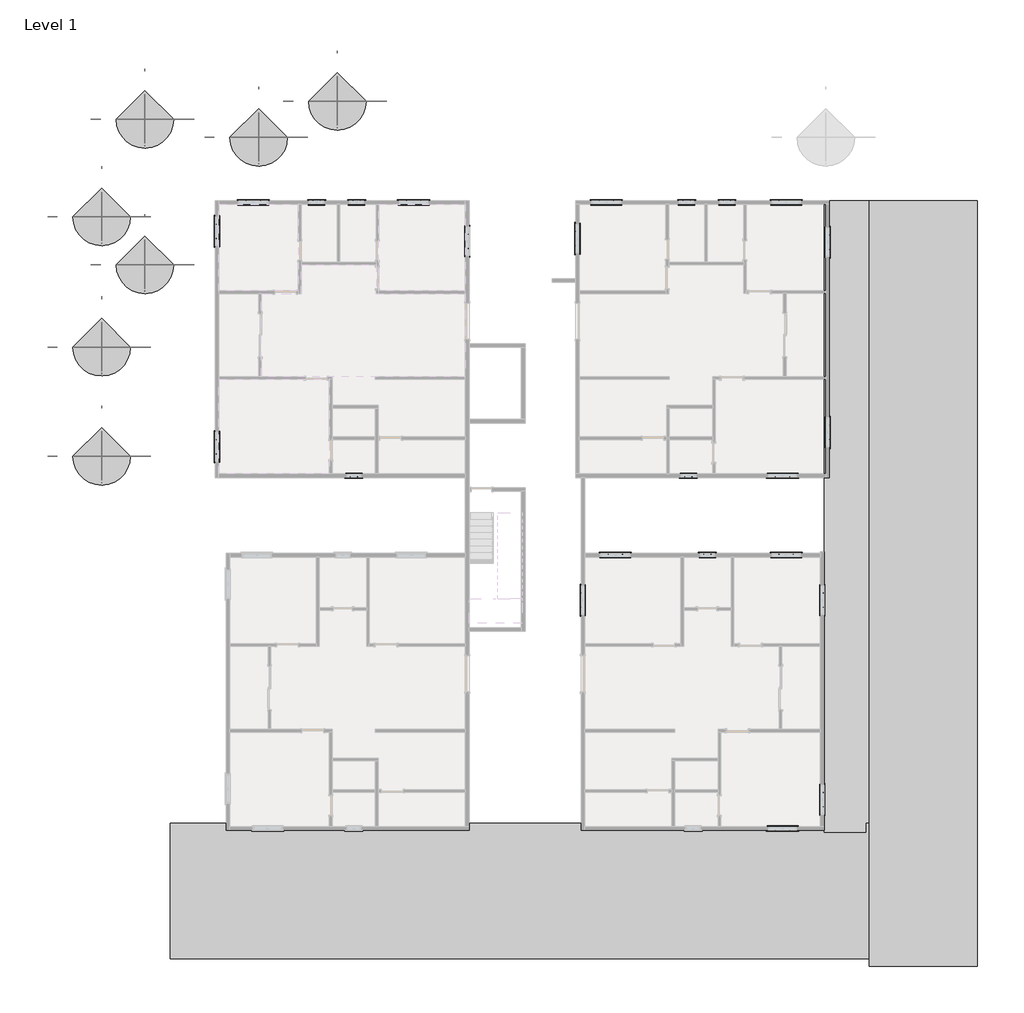
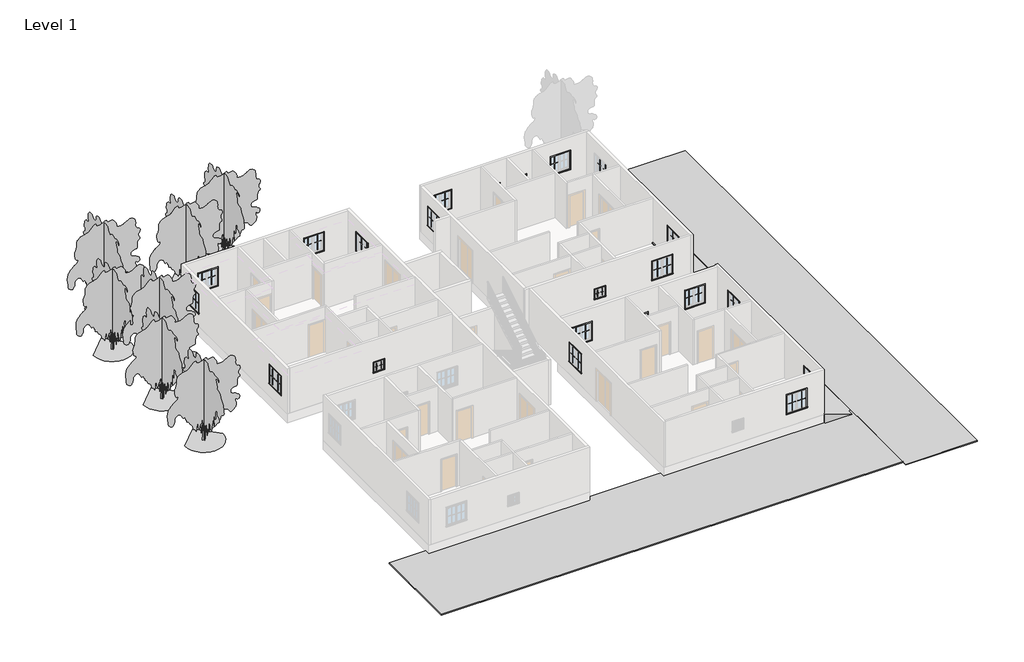
# One storey, part 6 of 7: 97 proxies, 7 geographic elements.
"""IFC4 building model written with IfcOpenShell, lengths in millimetres."""

from ifc_helpers import new_model, si_unit, origin, place, context, project, spatial, transform, mapped, element, save
from components import generic_models_1_generic_models_1_ebf34461, generic_models_2_generic_models_2_33b85b70, generic_models_3_generic_models_3_73c16d2e, muntin_pattern_2x2_muntin_pattern_2x2_4dfeb3f3, muntin_pattern_2x2_muntin_pattern_2x2_e852a7e4, muntin_pattern_2x2_muntin_pattern_2x2_0961b91c, muntin_pattern_2x2_muntin_pattern_2x2_cae9449b, trim_window_exterior_flat_with_sill_7cfdd449, trim_window_exterior_flat_with_sill_858dc10d, trim_window_interior_flat_picture_frame_f1e0b15b, trim_window_interior_flat_picture_frame_3927330c, rpc_tree_deciduous_golden_chain_18_92130817

model = new_model("IFC4")

# Units and contexts
model_context = context("Model", 3, world=origin())
ifc_project = project(units=[si_unit("LENGTHUNIT", "METRE", prefix="MILLI")], contexts=[model_context])

# Site, building, storey
site = spatial("IfcSite", under=ifc_project)
building = spatial("IfcBuilding", under=site)
storey = spatial("IfcBuildingStorey", under=building, Name="Level 1", Elevation=0.0)

# Proxies
placement = place(None, origin())
generic_models_1_generic_models_1_shape = generic_models_1_generic_models_1_ebf34461(model_context)
element("IfcBuildingElementProxy", 1, Name="Generic Models 1 : Generic Models 1", ObjectType="Generic Models 1 : Generic Models 1", at=placement, inside=storey, context=model_context, shape_type="MappedRepresentation", body=[
    mapped(generic_models_1_generic_models_1_shape, transform((0.0, 0.0, 0.0), x_axis=(1.0, 0.0, 0.0), y_axis=(0.0, 1.0, 0.0), z_axis=(0.0, 0.0, 1.0))),
])
generic_models_2_generic_models_2_shape = generic_models_2_generic_models_2_33b85b70(model_context)
element("IfcBuildingElementProxy", 2, Name="Generic Models 2 : Generic Models 2", ObjectType="Generic Models 2 : Generic Models 2", at=placement, inside=storey, context=model_context, shape_type="MappedRepresentation", body=[
    mapped(generic_models_2_generic_models_2_shape, transform((0.0, 0.0, 0.0), x_axis=(1.0, 0.0, 0.0), y_axis=(0.0, 1.0, 0.0), z_axis=(0.0, 0.0, 1.0))),
])
generic_models_3_generic_models_3_shape = generic_models_3_generic_models_3_73c16d2e(model_context)
element("IfcBuildingElementProxy", 3, Name="Generic Models 3 : Generic Models 3", ObjectType="Generic Models 3 : Generic Models 3", at=placement, inside=storey, context=model_context, shape_type="MappedRepresentation", body=[
    mapped(generic_models_3_generic_models_3_shape, transform((0.0, 0.0, 0.0), x_axis=(1.0, 0.0, 0.0), y_axis=(0.0, 1.0, 0.0), z_axis=(0.0, 0.0, 1.0))),
])
muntin_pattern_2x2_muntin_pattern_2x2_shape = muntin_pattern_2x2_muntin_pattern_2x2_4dfeb3f3(model_context)
element("IfcBuildingElementProxy", 4, Name="Muntin Pattern_2x2 : Muntin Pattern_2x2", ObjectType="Muntin Pattern_2x2 : Muntin Pattern_2x2", at=placement, inside=storey, context=model_context, shape_type="MappedRepresentation", body=[
    mapped(muntin_pattern_2x2_muntin_pattern_2x2_shape, transform((-12912.2969485, 13812.8685985, 984.25), x_axis=(1.0, 0.0, 0.0), y_axis=(0.0, 1.0, 0.0), z_axis=(0.0, 0.0, 1.0))),
])
element("IfcBuildingElementProxy", 5, Name="Muntin Pattern_2x2 : Muntin Pattern_2x2", ObjectType="Muntin Pattern_2x2 : Muntin Pattern_2x2", at=placement, inside=storey, context=model_context, shape_type="MappedRepresentation", body=[
    mapped(muntin_pattern_2x2_muntin_pattern_2x2_shape, transform((-14199.7594485, 12223.7810985, 984.25), x_axis=(0.0, 1.0, 0.0), y_axis=(-1.0, 0.0, 0.0), z_axis=(0.0, 0.0, 1.0))),
])
element("IfcBuildingElementProxy", 6, Name="Muntin Pattern_2x2 : Muntin Pattern_2x2", ObjectType="Muntin Pattern_2x2 : Muntin Pattern_2x2", at=placement, inside=storey, context=model_context, shape_type="MappedRepresentation", body=[
    mapped(muntin_pattern_2x2_muntin_pattern_2x2_shape, transform((-14199.7594485, 3130.5810985, 984.25), x_axis=(0.0, 1.0, 0.0), y_axis=(-1.0, 0.0, 0.0), z_axis=(0.0, 0.0, 1.0))),
])
element("IfcBuildingElementProxy", 7, Name="Muntin Pattern_2x2 : Muntin Pattern_2x2", ObjectType="Muntin Pattern_2x2 : Muntin Pattern_2x2", at=placement, inside=storey, context=model_context, shape_type="MappedRepresentation", body=[
    mapped(muntin_pattern_2x2_muntin_pattern_2x2_shape, transform((-6149.5469485, 13812.8685985, 984.25), x_axis=(1.0, 0.0, 0.0), y_axis=(0.0, 1.0, 0.0), z_axis=(0.0, 0.0, 1.0))),
])
element("IfcBuildingElementProxy", 8, Name="Muntin Pattern_2x2 : Muntin Pattern_2x2", ObjectType="Muntin Pattern_2x2 : Muntin Pattern_2x2", at=placement, inside=storey, context=model_context, shape_type="MappedRepresentation", body=[
    mapped(muntin_pattern_2x2_muntin_pattern_2x2_shape, transform((-3512.7094485, 12406.3051514, 984.25), x_axis=(0.0, -1.0, 0.0), y_axis=(1.0, 0.0, 0.0), z_axis=(0.0, 0.0, 1.0))),
])
element("IfcBuildingElementProxy", 9, Name="Muntin Pattern_2x2 : Muntin Pattern_2x2", ObjectType="Muntin Pattern_2x2 : Muntin Pattern_2x2", at=placement, inside=storey, context=model_context, shape_type="MappedRepresentation", body=[
    mapped(muntin_pattern_2x2_muntin_pattern_2x2_shape, transform((1002.2264317, 11918.9810985, 984.25), x_axis=(0.0, 1.0, 0.0), y_axis=(-1.0, 0.0, 0.0), z_axis=(0.0, 0.0, 1.0))),
])
element("IfcBuildingElementProxy", 10, Name="Muntin Pattern_2x2 : Muntin Pattern_2x2", ObjectType="Muntin Pattern_2x2 : Muntin Pattern_2x2", at=placement, inside=storey, context=model_context, shape_type="MappedRepresentation", body=[
    mapped(muntin_pattern_2x2_muntin_pattern_2x2_shape, transform((1984.8889317, 13812.8685985, 984.25), x_axis=(1.0, 0.0, 0.0), y_axis=(0.0, 1.0, 0.0), z_axis=(0.0, 0.0, 1.0))),
])
element("IfcBuildingElementProxy", 11, Name="Muntin Pattern_2x2 : Muntin Pattern_2x2", ObjectType="Muntin Pattern_2x2 : Muntin Pattern_2x2", at=placement, inside=storey, context=model_context, shape_type="MappedRepresentation", body=[
    mapped(muntin_pattern_2x2_muntin_pattern_2x2_shape, transform((9576.3139317, 13812.8685985, 984.25), x_axis=(1.0, 0.0, 0.0), y_axis=(0.0, 1.0, 0.0), z_axis=(0.0, 0.0, 1.0))),
])
element("IfcBuildingElementProxy", 12, Name="Muntin Pattern_2x2 : Muntin Pattern_2x2", ObjectType="Muntin Pattern_2x2 : Muntin Pattern_2x2", at=placement, inside=storey, context=model_context, shape_type="MappedRepresentation", body=[
    mapped(muntin_pattern_2x2_muntin_pattern_2x2_shape, transform((11689.2764317, 12373.0060985, 984.25), x_axis=(0.0, -1.0, 0.0), y_axis=(1.0, 0.0, 0.0), z_axis=(0.0, 0.0, 1.0))),
])
element("IfcBuildingElementProxy", 13, Name="Muntin Pattern_2x2 : Muntin Pattern_2x2", ObjectType="Muntin Pattern_2x2 : Muntin Pattern_2x2", at=placement, inside=storey, context=model_context, shape_type="MappedRepresentation", body=[
    mapped(muntin_pattern_2x2_muntin_pattern_2x2_shape, transform((10025.7910285, 2147.9185985, 984.25), x_axis=(-1.0, 0.0, 0.0), y_axis=(0.0, -1.0, 0.0), z_axis=(0.0, 0.0, 1.0))),
])
element("IfcBuildingElementProxy", 14, Name="Muntin Pattern_2x2 : Muntin Pattern_2x2", ObjectType="Muntin Pattern_2x2 : Muntin Pattern_2x2", at=placement, inside=storey, context=model_context, shape_type="MappedRepresentation", body=[
    mapped(muntin_pattern_2x2_muntin_pattern_2x2_shape, transform((11689.2764317, 4346.6060985, 984.25), x_axis=(0.0, -1.0, 0.0), y_axis=(1.0, 0.0, 0.0), z_axis=(0.0, 0.0, 1.0))),
])
element("IfcBuildingElementProxy", 15, Name="Muntin Pattern_2x2 : Muntin Pattern_2x2", ObjectType="Muntin Pattern_2x2 : Muntin Pattern_2x2", at=placement, inside=storey, context=model_context, shape_type="MappedRepresentation", body=[
    mapped(muntin_pattern_2x2_muntin_pattern_2x2_shape, transform((2365.8030515, -1071.5314015, 984.25), x_axis=(1.0, 0.0, 0.0), y_axis=(0.0, 1.0, 0.0), z_axis=(0.0, 0.0, 1.0))),
])
element("IfcBuildingElementProxy", 16, Name="Muntin Pattern_2x2 : Muntin Pattern_2x2", ObjectType="Muntin Pattern_2x2 : Muntin Pattern_2x2", at=placement, inside=storey, context=model_context, shape_type="MappedRepresentation", body=[
    mapped(muntin_pattern_2x2_muntin_pattern_2x2_shape, transform((1230.7405515, -3336.8939015, 984.25), x_axis=(0.0, 1.0, 0.0), y_axis=(-1.0, 0.0, 0.0), z_axis=(0.0, 0.0, 1.0))),
])
element("IfcBuildingElementProxy", 17, Name="Muntin Pattern_2x2 : Muntin Pattern_2x2", ObjectType="Muntin Pattern_2x2 : Muntin Pattern_2x2", at=placement, inside=storey, context=model_context, shape_type="MappedRepresentation", body=[
    mapped(muntin_pattern_2x2_muntin_pattern_2x2_shape, transform((9571.7660285, -1071.5314015, 984.25), x_axis=(1.0, 0.0, 0.0), y_axis=(0.0, 1.0, 0.0), z_axis=(0.0, 0.0, 1.0))),
])
element("IfcBuildingElementProxy", 18, Name="Muntin Pattern_2x2 : Muntin Pattern_2x2", ObjectType="Muntin Pattern_2x2 : Muntin Pattern_2x2", at=placement, inside=storey, context=model_context, shape_type="MappedRepresentation", body=[
    mapped(muntin_pattern_2x2_muntin_pattern_2x2_shape, transform((11465.6535285, -2730.4689015, 984.25), x_axis=(0.0, -1.0, 0.0), y_axis=(1.0, 0.0, 0.0), z_axis=(0.0, 0.0, 1.0))),
])
element("IfcBuildingElementProxy", 19, Name="Muntin Pattern_2x2 : Muntin Pattern_2x2", ObjectType="Muntin Pattern_2x2 : Muntin Pattern_2x2", at=placement, inside=storey, context=model_context, shape_type="MappedRepresentation", body=[
    mapped(muntin_pattern_2x2_muntin_pattern_2x2_shape, transform((11465.6535285, -11147.3939015, 984.25), x_axis=(0.0, -1.0, 0.0), y_axis=(1.0, 0.0, 0.0), z_axis=(0.0, 0.0, 1.0))),
])
element("IfcBuildingElementProxy", 20, Name="Muntin Pattern_2x2 : Muntin Pattern_2x2", ObjectType="Muntin Pattern_2x2 : Muntin Pattern_2x2", at=placement, inside=storey, context=model_context, shape_type="MappedRepresentation", body=[
    mapped(muntin_pattern_2x2_muntin_pattern_2x2_shape, transform((10025.7910285, -12736.4814015, 984.25), x_axis=(-1.0, 0.0, 0.0), y_axis=(0.0, -1.0, 0.0), z_axis=(0.0, 0.0, 1.0))),
])
muntin_pattern_2x2_muntin_pattern_2x2_2_shape = muntin_pattern_2x2_muntin_pattern_2x2_e852a7e4(model_context)
element("IfcBuildingElementProxy", 21, Name="Muntin Pattern_2x2 : Muntin Pattern_2x2", ObjectType="Muntin Pattern_2x2 : Muntin Pattern_2x2", at=placement, inside=storey, context=model_context, shape_type="MappedRepresentation", body=[
    mapped(muntin_pattern_2x2_muntin_pattern_2x2_2_shape, transform((-12305.8719485, 13812.8685985, 984.25), x_axis=(-1.0, 0.0, 0.0), y_axis=(0.0, -1.0, 0.0), z_axis=(0.0, 0.0, 1.0))),
])
element("IfcBuildingElementProxy", 22, Name="Muntin Pattern_2x2 : Muntin Pattern_2x2", ObjectType="Muntin Pattern_2x2 : Muntin Pattern_2x2", at=placement, inside=storey, context=model_context, shape_type="MappedRepresentation", body=[
    mapped(muntin_pattern_2x2_muntin_pattern_2x2_2_shape, transform((-14199.7594485, 12830.2060985, 984.25), x_axis=(0.0, -1.0, 0.0), y_axis=(1.0, 0.0, 0.0), z_axis=(0.0, 0.0, 1.0))),
])
element("IfcBuildingElementProxy", 23, Name="Muntin Pattern_2x2 : Muntin Pattern_2x2", ObjectType="Muntin Pattern_2x2 : Muntin Pattern_2x2", at=placement, inside=storey, context=model_context, shape_type="MappedRepresentation", body=[
    mapped(muntin_pattern_2x2_muntin_pattern_2x2_2_shape, transform((-14199.7594485, 3737.0060985, 984.25), x_axis=(0.0, -1.0, 0.0), y_axis=(1.0, 0.0, 0.0), z_axis=(0.0, 0.0, 1.0))),
])
element("IfcBuildingElementProxy", 24, Name="Muntin Pattern_2x2 : Muntin Pattern_2x2", ObjectType="Muntin Pattern_2x2 : Muntin Pattern_2x2", at=placement, inside=storey, context=model_context, shape_type="MappedRepresentation", body=[
    mapped(muntin_pattern_2x2_muntin_pattern_2x2_2_shape, transform((-5543.1219485, 13812.8685985, 984.25), x_axis=(-1.0, 0.0, 0.0), y_axis=(0.0, -1.0, 0.0), z_axis=(0.0, 0.0, 1.0))),
])
element("IfcBuildingElementProxy", 25, Name="Muntin Pattern_2x2 : Muntin Pattern_2x2", ObjectType="Muntin Pattern_2x2 : Muntin Pattern_2x2", at=placement, inside=storey, context=model_context, shape_type="MappedRepresentation", body=[
    mapped(muntin_pattern_2x2_muntin_pattern_2x2_2_shape, transform((-3512.7094485, 11799.8801514, 984.25), x_axis=(0.0, 1.0, 0.0), y_axis=(-1.0, 0.0, 0.0), z_axis=(0.0, 0.0, 1.0))),
])
element("IfcBuildingElementProxy", 26, Name="Muntin Pattern_2x2 : Muntin Pattern_2x2", ObjectType="Muntin Pattern_2x2 : Muntin Pattern_2x2", at=placement, inside=storey, context=model_context, shape_type="MappedRepresentation", body=[
    mapped(muntin_pattern_2x2_muntin_pattern_2x2_2_shape, transform((1002.2264317, 12525.4060985, 984.25), x_axis=(0.0, -1.0, 0.0), y_axis=(1.0, 0.0, 0.0), z_axis=(0.0, 0.0, 1.0))),
])
element("IfcBuildingElementProxy", 27, Name="Muntin Pattern_2x2 : Muntin Pattern_2x2", ObjectType="Muntin Pattern_2x2 : Muntin Pattern_2x2", at=placement, inside=storey, context=model_context, shape_type="MappedRepresentation", body=[
    mapped(muntin_pattern_2x2_muntin_pattern_2x2_2_shape, transform((2591.3139317, 13812.8685985, 984.25), x_axis=(-1.0, 0.0, 0.0), y_axis=(0.0, -1.0, 0.0), z_axis=(0.0, 0.0, 1.0))),
])
element("IfcBuildingElementProxy", 28, Name="Muntin Pattern_2x2 : Muntin Pattern_2x2", ObjectType="Muntin Pattern_2x2 : Muntin Pattern_2x2", at=placement, inside=storey, context=model_context, shape_type="MappedRepresentation", body=[
    mapped(muntin_pattern_2x2_muntin_pattern_2x2_2_shape, transform((11689.2764317, 11766.5810985, 984.25), x_axis=(0.0, 1.0, 0.0), y_axis=(-1.0, 0.0, 0.0), z_axis=(0.0, 0.0, 1.0))),
])
element("IfcBuildingElementProxy", 29, Name="Muntin Pattern_2x2 : Muntin Pattern_2x2", ObjectType="Muntin Pattern_2x2 : Muntin Pattern_2x2", at=placement, inside=storey, context=model_context, shape_type="MappedRepresentation", body=[
    mapped(muntin_pattern_2x2_muntin_pattern_2x2_2_shape, transform((9419.3660285, 2147.9185985, 984.25), x_axis=(1.0, 0.0, 0.0), y_axis=(0.0, 1.0, 0.0), z_axis=(0.0, 0.0, 1.0))),
])
element("IfcBuildingElementProxy", 30, Name="Muntin Pattern_2x2 : Muntin Pattern_2x2", ObjectType="Muntin Pattern_2x2 : Muntin Pattern_2x2", at=placement, inside=storey, context=model_context, shape_type="MappedRepresentation", body=[
    mapped(muntin_pattern_2x2_muntin_pattern_2x2_2_shape, transform((11689.2764317, 3740.1810985, 984.25), x_axis=(0.0, 1.0, 0.0), y_axis=(-1.0, 0.0, 0.0), z_axis=(0.0, 0.0, 1.0))),
])
element("IfcBuildingElementProxy", 31, Name="Muntin Pattern_2x2 : Muntin Pattern_2x2", ObjectType="Muntin Pattern_2x2 : Muntin Pattern_2x2", at=placement, inside=storey, context=model_context, shape_type="MappedRepresentation", body=[
    mapped(muntin_pattern_2x2_muntin_pattern_2x2_2_shape, transform((2972.2280515, -1071.5314015, 984.25), x_axis=(-1.0, 0.0, 0.0), y_axis=(0.0, -1.0, 0.0), z_axis=(0.0, 0.0, 1.0))),
])
element("IfcBuildingElementProxy", 32, Name="Muntin Pattern_2x2 : Muntin Pattern_2x2", ObjectType="Muntin Pattern_2x2 : Muntin Pattern_2x2", at=placement, inside=storey, context=model_context, shape_type="MappedRepresentation", body=[
    mapped(muntin_pattern_2x2_muntin_pattern_2x2_2_shape, transform((1230.7405515, -2730.4689015, 984.25), x_axis=(0.0, -1.0, 0.0), y_axis=(1.0, 0.0, 0.0), z_axis=(0.0, 0.0, 1.0))),
])
element("IfcBuildingElementProxy", 33, Name="Muntin Pattern_2x2 : Muntin Pattern_2x2", ObjectType="Muntin Pattern_2x2 : Muntin Pattern_2x2", at=placement, inside=storey, context=model_context, shape_type="MappedRepresentation", body=[
    mapped(muntin_pattern_2x2_muntin_pattern_2x2_2_shape, transform((10178.1910285, -1071.5314015, 984.25), x_axis=(-1.0, 0.0, 0.0), y_axis=(0.0, -1.0, 0.0), z_axis=(0.0, 0.0, 1.0))),
])
element("IfcBuildingElementProxy", 34, Name="Muntin Pattern_2x2 : Muntin Pattern_2x2", ObjectType="Muntin Pattern_2x2 : Muntin Pattern_2x2", at=placement, inside=storey, context=model_context, shape_type="MappedRepresentation", body=[
    mapped(muntin_pattern_2x2_muntin_pattern_2x2_2_shape, transform((11465.6535285, -3336.8939015, 984.25), x_axis=(0.0, 1.0, 0.0), y_axis=(-1.0, 0.0, 0.0), z_axis=(0.0, 0.0, 1.0))),
])
element("IfcBuildingElementProxy", 35, Name="Muntin Pattern_2x2 : Muntin Pattern_2x2", ObjectType="Muntin Pattern_2x2 : Muntin Pattern_2x2", at=placement, inside=storey, context=model_context, shape_type="MappedRepresentation", body=[
    mapped(muntin_pattern_2x2_muntin_pattern_2x2_2_shape, transform((11465.6535285, -11753.8189015, 984.25), x_axis=(0.0, 1.0, 0.0), y_axis=(-1.0, 0.0, 0.0), z_axis=(0.0, 0.0, 1.0))),
])
element("IfcBuildingElementProxy", 36, Name="Muntin Pattern_2x2 : Muntin Pattern_2x2", ObjectType="Muntin Pattern_2x2 : Muntin Pattern_2x2", at=placement, inside=storey, context=model_context, shape_type="MappedRepresentation", body=[
    mapped(muntin_pattern_2x2_muntin_pattern_2x2_2_shape, transform((9419.3660285, -12736.4814015, 984.25), x_axis=(1.0, 0.0, 0.0), y_axis=(0.0, 1.0, 0.0), z_axis=(0.0, 0.0, 1.0))),
])
muntin_pattern_2x2_muntin_pattern_2x2_3_shape = muntin_pattern_2x2_muntin_pattern_2x2_0961b91c(model_context)
element("IfcBuildingElementProxy", 37, Name="Muntin Pattern_2x2 : Muntin Pattern_2x2", ObjectType="Muntin Pattern_2x2 : Muntin Pattern_2x2", at=placement, inside=storey, context=model_context, shape_type="MappedRepresentation", body=[
    mapped(muntin_pattern_2x2_muntin_pattern_2x2_3_shape, transform((-10086.5469485, 13812.8685985, 984.25), x_axis=(1.0, 0.0, 0.0), y_axis=(0.0, 1.0, 0.0), z_axis=(0.0, 0.0, 1.0))),
])
element("IfcBuildingElementProxy", 38, Name="Muntin Pattern_2x2 : Muntin Pattern_2x2", ObjectType="Muntin Pattern_2x2 : Muntin Pattern_2x2", at=placement, inside=storey, context=model_context, shape_type="MappedRepresentation", body=[
    mapped(muntin_pattern_2x2_muntin_pattern_2x2_3_shape, transform((-8397.4469485, 13812.8685985, 984.25), x_axis=(1.0, 0.0, 0.0), y_axis=(0.0, 1.0, 0.0), z_axis=(0.0, 0.0, 1.0))),
])
element("IfcBuildingElementProxy", 39, Name="Muntin Pattern_2x2 : Muntin Pattern_2x2", ObjectType="Muntin Pattern_2x2 : Muntin Pattern_2x2", at=placement, inside=storey, context=model_context, shape_type="MappedRepresentation", body=[
    mapped(muntin_pattern_2x2_muntin_pattern_2x2_3_shape, transform((-8216.4719485, 2147.9185985, 984.25), x_axis=(-1.0, 0.0, 0.0), y_axis=(0.0, -1.0, 0.0), z_axis=(0.0, 0.0, 1.0))),
])
element("IfcBuildingElementProxy", 40, Name="Muntin Pattern_2x2 : Muntin Pattern_2x2", ObjectType="Muntin Pattern_2x2 : Muntin Pattern_2x2", at=placement, inside=storey, context=model_context, shape_type="MappedRepresentation", body=[
    mapped(muntin_pattern_2x2_muntin_pattern_2x2_3_shape, transform((6396.7660285, -1071.5314015, 984.25), x_axis=(1.0, 0.0, 0.0), y_axis=(0.0, 1.0, 0.0), z_axis=(0.0, 0.0, 1.0))),
])
element("IfcBuildingElementProxy", 41, Name="Muntin Pattern_2x2 : Muntin Pattern_2x2", ObjectType="Muntin Pattern_2x2 : Muntin Pattern_2x2", at=placement, inside=storey, context=model_context, shape_type="MappedRepresentation", body=[
    mapped(muntin_pattern_2x2_muntin_pattern_2x2_3_shape, transform((5899.6639317, 2147.9185985, 984.25), x_axis=(-1.0, 0.0, 0.0), y_axis=(0.0, -1.0, 0.0), z_axis=(0.0, 0.0, 1.0))),
])
element("IfcBuildingElementProxy", 42, Name="Muntin Pattern_2x2 : Muntin Pattern_2x2", ObjectType="Muntin Pattern_2x2 : Muntin Pattern_2x2", at=placement, inside=storey, context=model_context, shape_type="MappedRepresentation", body=[
    mapped(muntin_pattern_2x2_muntin_pattern_2x2_3_shape, transform((5528.1889317, 13812.8685985, 984.25), x_axis=(1.0, 0.0, 0.0), y_axis=(0.0, 1.0, 0.0), z_axis=(0.0, 0.0, 1.0))),
])
element("IfcBuildingElementProxy", 43, Name="Muntin Pattern_2x2 : Muntin Pattern_2x2", ObjectType="Muntin Pattern_2x2 : Muntin Pattern_2x2", at=placement, inside=storey, context=model_context, shape_type="MappedRepresentation", body=[
    mapped(muntin_pattern_2x2_muntin_pattern_2x2_3_shape, transform((7223.6389317, 13812.8685985, 984.25), x_axis=(1.0, 0.0, 0.0), y_axis=(0.0, 1.0, 0.0), z_axis=(0.0, 0.0, 1.0))),
])
muntin_pattern_2x2_muntin_pattern_2x2_4_shape = muntin_pattern_2x2_muntin_pattern_2x2_cae9449b(model_context)
element("IfcBuildingElementProxy", 44, Name="Muntin Pattern_2x2 : Muntin Pattern_2x2", ObjectType="Muntin Pattern_2x2 : Muntin Pattern_2x2", at=placement, inside=storey, context=model_context, shape_type="MappedRepresentation", body=[
    mapped(muntin_pattern_2x2_muntin_pattern_2x2_4_shape, transform((-9784.9219485, 13812.8685985, 984.25), x_axis=(-1.0, 0.0, 0.0), y_axis=(0.0, -1.0, 0.0), z_axis=(0.0, 0.0, 1.0))),
])
element("IfcBuildingElementProxy", 45, Name="Muntin Pattern_2x2 : Muntin Pattern_2x2", ObjectType="Muntin Pattern_2x2 : Muntin Pattern_2x2", at=placement, inside=storey, context=model_context, shape_type="MappedRepresentation", body=[
    mapped(muntin_pattern_2x2_muntin_pattern_2x2_4_shape, transform((-8095.8219485, 13812.8685985, 984.25), x_axis=(-1.0, 0.0, 0.0), y_axis=(0.0, -1.0, 0.0), z_axis=(0.0, 0.0, 1.0))),
])
element("IfcBuildingElementProxy", 46, Name="Muntin Pattern_2x2 : Muntin Pattern_2x2", ObjectType="Muntin Pattern_2x2 : Muntin Pattern_2x2", at=placement, inside=storey, context=model_context, shape_type="MappedRepresentation", body=[
    mapped(muntin_pattern_2x2_muntin_pattern_2x2_4_shape, transform((-8518.0969485, 2147.9185985, 984.25), x_axis=(1.0, 0.0, 0.0), y_axis=(0.0, 1.0, 0.0), z_axis=(0.0, 0.0, 1.0))),
])
element("IfcBuildingElementProxy", 47, Name="Muntin Pattern_2x2 : Muntin Pattern_2x2", ObjectType="Muntin Pattern_2x2 : Muntin Pattern_2x2", at=placement, inside=storey, context=model_context, shape_type="MappedRepresentation", body=[
    mapped(muntin_pattern_2x2_muntin_pattern_2x2_4_shape, transform((6698.3910285, -1071.5314015, 984.25), x_axis=(-1.0, 0.0, 0.0), y_axis=(0.0, -1.0, 0.0), z_axis=(0.0, 0.0, 1.0))),
])
element("IfcBuildingElementProxy", 48, Name="Muntin Pattern_2x2 : Muntin Pattern_2x2", ObjectType="Muntin Pattern_2x2 : Muntin Pattern_2x2", at=placement, inside=storey, context=model_context, shape_type="MappedRepresentation", body=[
    mapped(muntin_pattern_2x2_muntin_pattern_2x2_4_shape, transform((5598.0389317, 2147.9185985, 984.25), x_axis=(1.0, 0.0, 0.0), y_axis=(0.0, 1.0, 0.0), z_axis=(0.0, 0.0, 1.0))),
])
element("IfcBuildingElementProxy", 49, Name="Muntin Pattern_2x2 : Muntin Pattern_2x2", ObjectType="Muntin Pattern_2x2 : Muntin Pattern_2x2", at=placement, inside=storey, context=model_context, shape_type="MappedRepresentation", body=[
    mapped(muntin_pattern_2x2_muntin_pattern_2x2_4_shape, transform((5829.8139317, 13812.8685985, 984.25), x_axis=(-1.0, 0.0, 0.0), y_axis=(0.0, -1.0, 0.0), z_axis=(0.0, 0.0, 1.0))),
])
element("IfcBuildingElementProxy", 50, Name="Muntin Pattern_2x2 : Muntin Pattern_2x2", ObjectType="Muntin Pattern_2x2 : Muntin Pattern_2x2", at=placement, inside=storey, context=model_context, shape_type="MappedRepresentation", body=[
    mapped(muntin_pattern_2x2_muntin_pattern_2x2_4_shape, transform((7525.2639317, 13812.8685985, 984.25), x_axis=(-1.0, 0.0, 0.0), y_axis=(0.0, -1.0, 0.0), z_axis=(0.0, 0.0, 1.0))),
])
trim_window_exterior_flat_with_sill_shape = trim_window_exterior_flat_with_sill_7cfdd449(model_context)
element("IfcBuildingElementProxy", 51, Name="Trim-Window-Exterior-Flat : with Sill", ObjectType="Trim-Window-Exterior-Flat : with Sill", at=placement, inside=storey, context=model_context, shape_type="MappedRepresentation", body=[
    mapped(trim_window_exterior_flat_with_sill_shape, transform((-12609.0844485, 13822.3935985, 2133.6), x_axis=(-1.0, 0.0, 0.0), y_axis=(0.0, 0.0, 1.0), z_axis=(0.0, 1.0, 0.0))),
])
element("IfcBuildingElementProxy", 52, Name="Trim-Window-Exterior-Flat : with Sill", ObjectType="Trim-Window-Exterior-Flat : with Sill", at=placement, inside=storey, context=model_context, shape_type="MappedRepresentation", body=[
    mapped(trim_window_exterior_flat_with_sill_shape, transform((-14209.2844485, 12526.9935985, 2133.6), x_axis=(0.0, -1.0, 0.0), y_axis=(0.0, 0.0, 1.0), z_axis=(-1.0, 0.0, 0.0))),
])
element("IfcBuildingElementProxy", 53, Name="Trim-Window-Exterior-Flat : with Sill", ObjectType="Trim-Window-Exterior-Flat : with Sill", at=placement, inside=storey, context=model_context, shape_type="MappedRepresentation", body=[
    mapped(trim_window_exterior_flat_with_sill_shape, transform((-14209.2844485, 3433.7935985, 2133.6), x_axis=(0.0, -1.0, 0.0), y_axis=(0.0, 0.0, 1.0), z_axis=(-1.0, 0.0, 0.0))),
])
element("IfcBuildingElementProxy", 54, Name="Trim-Window-Exterior-Flat : with Sill", ObjectType="Trim-Window-Exterior-Flat : with Sill", at=placement, inside=storey, context=model_context, shape_type="MappedRepresentation", body=[
    mapped(trim_window_exterior_flat_with_sill_shape, transform((-5846.3344485, 13822.3935985, 2133.6), x_axis=(-1.0, 0.0, 0.0), y_axis=(0.0, 0.0, 1.0), z_axis=(0.0, 1.0, 0.0))),
])
element("IfcBuildingElementProxy", 55, Name="Trim-Window-Exterior-Flat : with Sill", ObjectType="Trim-Window-Exterior-Flat : with Sill", at=placement, inside=storey, context=model_context, shape_type="MappedRepresentation", body=[
    mapped(trim_window_exterior_flat_with_sill_shape, transform((-3503.1844485, 12103.0926514, 2133.6), x_axis=(0.0, 1.0, 0.0), y_axis=(0.0, 0.0, 1.0), z_axis=(1.0, 0.0, 0.0))),
])
element("IfcBuildingElementProxy", 56, Name="Trim-Window-Exterior-Flat : with Sill", ObjectType="Trim-Window-Exterior-Flat : with Sill", at=placement, inside=storey, context=model_context, shape_type="MappedRepresentation", body=[
    mapped(trim_window_exterior_flat_with_sill_shape, transform((992.7014317, 12222.1935985, 2133.6), x_axis=(0.0, -1.0, 0.0), y_axis=(0.0, 0.0, 1.0), z_axis=(-1.0, 0.0, 0.0))),
])
element("IfcBuildingElementProxy", 57, Name="Trim-Window-Exterior-Flat : with Sill", ObjectType="Trim-Window-Exterior-Flat : with Sill", at=placement, inside=storey, context=model_context, shape_type="MappedRepresentation", body=[
    mapped(trim_window_exterior_flat_with_sill_shape, transform((2288.1014317, 13822.3935985, 2133.6), x_axis=(-1.0, 0.0, 0.0), y_axis=(0.0, 0.0, 1.0), z_axis=(0.0, 1.0, 0.0))),
])
element("IfcBuildingElementProxy", 58, Name="Trim-Window-Exterior-Flat : with Sill", ObjectType="Trim-Window-Exterior-Flat : with Sill", at=placement, inside=storey, context=model_context, shape_type="MappedRepresentation", body=[
    mapped(trim_window_exterior_flat_with_sill_shape, transform((9879.5264317, 13822.3935985, 2133.6), x_axis=(-1.0, 0.0, 0.0), y_axis=(0.0, 0.0, 1.0), z_axis=(0.0, 1.0, 0.0))),
])
element("IfcBuildingElementProxy", 59, Name="Trim-Window-Exterior-Flat : with Sill", ObjectType="Trim-Window-Exterior-Flat : with Sill", at=placement, inside=storey, context=model_context, shape_type="MappedRepresentation", body=[
    mapped(trim_window_exterior_flat_with_sill_shape, transform((11698.8014317, 12069.7935985, 2133.6), x_axis=(0.0, 1.0, 0.0), y_axis=(0.0, 0.0, 1.0), z_axis=(1.0, 0.0, 0.0))),
])
element("IfcBuildingElementProxy", 60, Name="Trim-Window-Exterior-Flat : with Sill", ObjectType="Trim-Window-Exterior-Flat : with Sill", at=placement, inside=storey, context=model_context, shape_type="MappedRepresentation", body=[
    mapped(trim_window_exterior_flat_with_sill_shape, transform((9722.5785285, 2138.3935985, 2133.6), x_axis=(1.0, 0.0, 0.0), y_axis=(0.0, 0.0, 1.0), z_axis=(0.0, -1.0, 0.0))),
])
element("IfcBuildingElementProxy", 61, Name="Trim-Window-Exterior-Flat : with Sill", ObjectType="Trim-Window-Exterior-Flat : with Sill", at=placement, inside=storey, context=model_context, shape_type="MappedRepresentation", body=[
    mapped(trim_window_exterior_flat_with_sill_shape, transform((11698.8014317, 4043.3935985, 2133.6), x_axis=(0.0, 1.0, 0.0), y_axis=(0.0, 0.0, 1.0), z_axis=(1.0, 0.0, 0.0))),
])
element("IfcBuildingElementProxy", 62, Name="Trim-Window-Exterior-Flat : with Sill", ObjectType="Trim-Window-Exterior-Flat : with Sill", at=placement, inside=storey, context=model_context, shape_type="MappedRepresentation", body=[
    mapped(trim_window_exterior_flat_with_sill_shape, transform((2669.0155515, -1062.0064015, 2133.6), x_axis=(-1.0, 0.0, 0.0), y_axis=(0.0, 0.0, 1.0), z_axis=(0.0, 1.0, 0.0))),
])
element("IfcBuildingElementProxy", 63, Name="Trim-Window-Exterior-Flat : with Sill", ObjectType="Trim-Window-Exterior-Flat : with Sill", at=placement, inside=storey, context=model_context, shape_type="MappedRepresentation", body=[
    mapped(trim_window_exterior_flat_with_sill_shape, transform((1221.2155515, -3033.6814015, 2133.6), x_axis=(0.0, -1.0, 0.0), y_axis=(0.0, 0.0, 1.0), z_axis=(-1.0, 0.0, 0.0))),
])
element("IfcBuildingElementProxy", 64, Name="Trim-Window-Exterior-Flat : with Sill", ObjectType="Trim-Window-Exterior-Flat : with Sill", at=placement, inside=storey, context=model_context, shape_type="MappedRepresentation", body=[
    mapped(trim_window_exterior_flat_with_sill_shape, transform((9874.9785285, -1062.0064015, 2133.6), x_axis=(-1.0, 0.0, 0.0), y_axis=(0.0, 0.0, 1.0), z_axis=(0.0, 1.0, 0.0))),
])
element("IfcBuildingElementProxy", 65, Name="Trim-Window-Exterior-Flat : with Sill", ObjectType="Trim-Window-Exterior-Flat : with Sill", at=placement, inside=storey, context=model_context, shape_type="MappedRepresentation", body=[
    mapped(trim_window_exterior_flat_with_sill_shape, transform((11475.1785285, -3033.6814015, 2133.6), x_axis=(0.0, 1.0, 0.0), y_axis=(0.0, 0.0, 1.0), z_axis=(1.0, 0.0, 0.0))),
])
element("IfcBuildingElementProxy", 66, Name="Trim-Window-Exterior-Flat : with Sill", ObjectType="Trim-Window-Exterior-Flat : with Sill", at=placement, inside=storey, context=model_context, shape_type="MappedRepresentation", body=[
    mapped(trim_window_exterior_flat_with_sill_shape, transform((11475.1785285, -11450.6064015, 2133.6), x_axis=(0.0, 1.0, 0.0), y_axis=(0.0, 0.0, 1.0), z_axis=(1.0, 0.0, 0.0))),
])
element("IfcBuildingElementProxy", 67, Name="Trim-Window-Exterior-Flat : with Sill", ObjectType="Trim-Window-Exterior-Flat : with Sill", at=placement, inside=storey, context=model_context, shape_type="MappedRepresentation", body=[
    mapped(trim_window_exterior_flat_with_sill_shape, transform((9722.5785285, -12746.0064015, 2133.6), x_axis=(1.0, 0.0, 0.0), y_axis=(0.0, 0.0, 1.0), z_axis=(0.0, -1.0, 0.0))),
])
trim_window_exterior_flat_with_sill_2_shape = trim_window_exterior_flat_with_sill_858dc10d(model_context)
element("IfcBuildingElementProxy", 68, Name="Trim-Window-Exterior-Flat : with Sill", ObjectType="Trim-Window-Exterior-Flat : with Sill", at=placement, inside=storey, context=model_context, shape_type="MappedRepresentation", body=[
    mapped(trim_window_exterior_flat_with_sill_2_shape, transform((-9935.7344485, 13822.3935985, 1524.0), x_axis=(-1.0, 0.0, 0.0), y_axis=(0.0, 0.0, 1.0), z_axis=(0.0, 1.0, 0.0))),
])
element("IfcBuildingElementProxy", 69, Name="Trim-Window-Exterior-Flat : with Sill", ObjectType="Trim-Window-Exterior-Flat : with Sill", at=placement, inside=storey, context=model_context, shape_type="MappedRepresentation", body=[
    mapped(trim_window_exterior_flat_with_sill_2_shape, transform((-8246.6344485, 13822.3935985, 1524.0), x_axis=(-1.0, 0.0, 0.0), y_axis=(0.0, 0.0, 1.0), z_axis=(0.0, 1.0, 0.0))),
])
element("IfcBuildingElementProxy", 70, Name="Trim-Window-Exterior-Flat : with Sill", ObjectType="Trim-Window-Exterior-Flat : with Sill", at=placement, inside=storey, context=model_context, shape_type="MappedRepresentation", body=[
    mapped(trim_window_exterior_flat_with_sill_2_shape, transform((-8367.2844485, 2138.3935985, 1524.0), x_axis=(1.0, 0.0, 0.0), y_axis=(0.0, 0.0, 1.0), z_axis=(0.0, -1.0, 0.0))),
])
element("IfcBuildingElementProxy", 71, Name="Trim-Window-Exterior-Flat : with Sill", ObjectType="Trim-Window-Exterior-Flat : with Sill", at=placement, inside=storey, context=model_context, shape_type="MappedRepresentation", body=[
    mapped(trim_window_exterior_flat_with_sill_2_shape, transform((6547.5785285, -1062.0064015, 1524.0), x_axis=(-1.0, 0.0, 0.0), y_axis=(0.0, 0.0, 1.0), z_axis=(0.0, 1.0, 0.0))),
])
element("IfcBuildingElementProxy", 72, Name="Trim-Window-Exterior-Flat : with Sill", ObjectType="Trim-Window-Exterior-Flat : with Sill", at=placement, inside=storey, context=model_context, shape_type="MappedRepresentation", body=[
    mapped(trim_window_exterior_flat_with_sill_2_shape, transform((5748.8514317, 2138.3935985, 1524.0), x_axis=(1.0, 0.0, 0.0), y_axis=(0.0, 0.0, 1.0), z_axis=(0.0, -1.0, 0.0))),
])
element("IfcBuildingElementProxy", 73, Name="Trim-Window-Exterior-Flat : with Sill", ObjectType="Trim-Window-Exterior-Flat : with Sill", at=placement, inside=storey, context=model_context, shape_type="MappedRepresentation", body=[
    mapped(trim_window_exterior_flat_with_sill_2_shape, transform((5679.0014317, 13822.3935985, 1524.0), x_axis=(-1.0, 0.0, 0.0), y_axis=(0.0, 0.0, 1.0), z_axis=(0.0, 1.0, 0.0))),
])
element("IfcBuildingElementProxy", 74, Name="Trim-Window-Exterior-Flat : with Sill", ObjectType="Trim-Window-Exterior-Flat : with Sill", at=placement, inside=storey, context=model_context, shape_type="MappedRepresentation", body=[
    mapped(trim_window_exterior_flat_with_sill_2_shape, transform((7374.4514317, 13822.3935985, 1524.0), x_axis=(-1.0, 0.0, 0.0), y_axis=(0.0, 0.0, 1.0), z_axis=(0.0, 1.0, 0.0))),
])
trim_window_interior_flat_picture_frame_shape = trim_window_interior_flat_picture_frame_f1e0b15b(model_context)
element("IfcBuildingElementProxy", 75, Name="Trim-Window-Interior-Flat : Picture Frame", ObjectType="Trim-Window-Interior-Flat : Picture Frame", at=placement, inside=storey, context=model_context, shape_type="MappedRepresentation", body=[
    mapped(trim_window_interior_flat_picture_frame_shape, transform((-12609.0844485, 13669.9935985, 2133.6), x_axis=(1.0, 0.0, 0.0), y_axis=(0.0, 0.0, 1.0), z_axis=(0.0, -1.0, 0.0))),
])
element("IfcBuildingElementProxy", 76, Name="Trim-Window-Interior-Flat : Picture Frame", ObjectType="Trim-Window-Interior-Flat : Picture Frame", at=placement, inside=storey, context=model_context, shape_type="MappedRepresentation", body=[
    mapped(trim_window_interior_flat_picture_frame_shape, transform((-14056.8844485, 12526.9935985, 2133.6), x_axis=(0.0, 1.0, 0.0), y_axis=(0.0, 0.0, 1.0), z_axis=(1.0, 0.0, 0.0))),
])
element("IfcBuildingElementProxy", 77, Name="Trim-Window-Interior-Flat : Picture Frame", ObjectType="Trim-Window-Interior-Flat : Picture Frame", at=placement, inside=storey, context=model_context, shape_type="MappedRepresentation", body=[
    mapped(trim_window_interior_flat_picture_frame_shape, transform((-14056.8844485, 3433.7935985, 2133.6), x_axis=(0.0, 1.0, 0.0), y_axis=(0.0, 0.0, 1.0), z_axis=(1.0, 0.0, 0.0))),
])
element("IfcBuildingElementProxy", 78, Name="Trim-Window-Interior-Flat : Picture Frame", ObjectType="Trim-Window-Interior-Flat : Picture Frame", at=placement, inside=storey, context=model_context, shape_type="MappedRepresentation", body=[
    mapped(trim_window_interior_flat_picture_frame_shape, transform((-5846.3344485, 13669.9935985, 2133.6), x_axis=(1.0, 0.0, 0.0), y_axis=(0.0, 0.0, 1.0), z_axis=(0.0, -1.0, 0.0))),
])
element("IfcBuildingElementProxy", 79, Name="Trim-Window-Interior-Flat : Picture Frame", ObjectType="Trim-Window-Interior-Flat : Picture Frame", at=placement, inside=storey, context=model_context, shape_type="MappedRepresentation", body=[
    mapped(trim_window_interior_flat_picture_frame_shape, transform((-3655.5844485, 12103.0926514, 2133.6), x_axis=(0.0, -1.0, 0.0), y_axis=(0.0, 0.0, 1.0), z_axis=(-1.0, 0.0, 0.0))),
])
element("IfcBuildingElementProxy", 80, Name="Trim-Window-Interior-Flat : Picture Frame", ObjectType="Trim-Window-Interior-Flat : Picture Frame", at=placement, inside=storey, context=model_context, shape_type="MappedRepresentation", body=[
    mapped(trim_window_interior_flat_picture_frame_shape, transform((1145.1014317, 12222.1935985, 2133.6), x_axis=(0.0, 1.0, 0.0), y_axis=(0.0, 0.0, 1.0), z_axis=(1.0, 0.0, 0.0))),
])
element("IfcBuildingElementProxy", 81, Name="Trim-Window-Interior-Flat : Picture Frame", ObjectType="Trim-Window-Interior-Flat : Picture Frame", at=placement, inside=storey, context=model_context, shape_type="MappedRepresentation", body=[
    mapped(trim_window_interior_flat_picture_frame_shape, transform((2288.1014317, 13669.9935985, 2133.6), x_axis=(1.0, 0.0, 0.0), y_axis=(0.0, 0.0, 1.0), z_axis=(0.0, -1.0, 0.0))),
])
element("IfcBuildingElementProxy", 82, Name="Trim-Window-Interior-Flat : Picture Frame", ObjectType="Trim-Window-Interior-Flat : Picture Frame", at=placement, inside=storey, context=model_context, shape_type="MappedRepresentation", body=[
    mapped(trim_window_interior_flat_picture_frame_shape, transform((9879.5264317, 13669.9935985, 2133.6), x_axis=(1.0, 0.0, 0.0), y_axis=(0.0, 0.0, 1.0), z_axis=(0.0, -1.0, 0.0))),
])
element("IfcBuildingElementProxy", 83, Name="Trim-Window-Interior-Flat : Picture Frame", ObjectType="Trim-Window-Interior-Flat : Picture Frame", at=placement, inside=storey, context=model_context, shape_type="MappedRepresentation", body=[
    mapped(trim_window_interior_flat_picture_frame_shape, transform((9722.5785285, 2290.7935985, 2133.6), x_axis=(-1.0, 0.0, 0.0), y_axis=(0.0, 0.0, 1.0), z_axis=(0.0, 1.0, 0.0))),
])
element("IfcBuildingElementProxy", 84, Name="Trim-Window-Interior-Flat : Picture Frame", ObjectType="Trim-Window-Interior-Flat : Picture Frame", at=placement, inside=storey, context=model_context, shape_type="MappedRepresentation", body=[
    mapped(trim_window_interior_flat_picture_frame_shape, transform((11546.4014317, 4043.3935985, 2133.6), x_axis=(0.0, -1.0, 0.0), y_axis=(0.0, 0.0, 1.0), z_axis=(-1.0, 0.0, 0.0))),
])
element("IfcBuildingElementProxy", 85, Name="Trim-Window-Interior-Flat : Picture Frame", ObjectType="Trim-Window-Interior-Flat : Picture Frame", at=placement, inside=storey, context=model_context, shape_type="MappedRepresentation", body=[
    mapped(trim_window_interior_flat_picture_frame_shape, transform((2669.0155515, -1214.4064015, 2133.6), x_axis=(1.0, 0.0, 0.0), y_axis=(0.0, 0.0, 1.0), z_axis=(0.0, -1.0, 0.0))),
])
element("IfcBuildingElementProxy", 86, Name="Trim-Window-Interior-Flat : Picture Frame", ObjectType="Trim-Window-Interior-Flat : Picture Frame", at=placement, inside=storey, context=model_context, shape_type="MappedRepresentation", body=[
    mapped(trim_window_interior_flat_picture_frame_shape, transform((1373.6155515, -3033.6814015, 2133.6), x_axis=(0.0, 1.0, 0.0), y_axis=(0.0, 0.0, 1.0), z_axis=(1.0, 0.0, 0.0))),
])
element("IfcBuildingElementProxy", 87, Name="Trim-Window-Interior-Flat : Picture Frame", ObjectType="Trim-Window-Interior-Flat : Picture Frame", at=placement, inside=storey, context=model_context, shape_type="MappedRepresentation", body=[
    mapped(trim_window_interior_flat_picture_frame_shape, transform((9874.9785285, -1214.4064015, 2133.6), x_axis=(1.0, 0.0, 0.0), y_axis=(0.0, 0.0, 1.0), z_axis=(0.0, -1.0, 0.0))),
])
element("IfcBuildingElementProxy", 88, Name="Trim-Window-Interior-Flat : Picture Frame", ObjectType="Trim-Window-Interior-Flat : Picture Frame", at=placement, inside=storey, context=model_context, shape_type="MappedRepresentation", body=[
    mapped(trim_window_interior_flat_picture_frame_shape, transform((11322.7785285, -3033.6814015, 2133.6), x_axis=(0.0, -1.0, 0.0), y_axis=(0.0, 0.0, 1.0), z_axis=(-1.0, 0.0, 0.0))),
])
element("IfcBuildingElementProxy", 89, Name="Trim-Window-Interior-Flat : Picture Frame", ObjectType="Trim-Window-Interior-Flat : Picture Frame", at=placement, inside=storey, context=model_context, shape_type="MappedRepresentation", body=[
    mapped(trim_window_interior_flat_picture_frame_shape, transform((11322.7785285, -11450.6064015, 2133.6), x_axis=(0.0, -1.0, 0.0), y_axis=(0.0, 0.0, 1.0), z_axis=(-1.0, 0.0, 0.0))),
])
element("IfcBuildingElementProxy", 90, Name="Trim-Window-Interior-Flat : Picture Frame", ObjectType="Trim-Window-Interior-Flat : Picture Frame", at=placement, inside=storey, context=model_context, shape_type="MappedRepresentation", body=[
    mapped(trim_window_interior_flat_picture_frame_shape, transform((9722.5785285, -12593.6064015, 2133.6), x_axis=(-1.0, 0.0, 0.0), y_axis=(0.0, 0.0, 1.0), z_axis=(0.0, 1.0, 0.0))),
])
trim_window_interior_flat_picture_frame_2_shape = trim_window_interior_flat_picture_frame_3927330c(model_context)
element("IfcBuildingElementProxy", 91, Name="Trim-Window-Interior-Flat : Picture Frame", ObjectType="Trim-Window-Interior-Flat : Picture Frame", at=placement, inside=storey, context=model_context, shape_type="MappedRepresentation", body=[
    mapped(trim_window_interior_flat_picture_frame_2_shape, transform((-9935.7344485, 13669.9935985, 1524.0), x_axis=(1.0, 0.0, 0.0), y_axis=(0.0, 0.0, 1.0), z_axis=(0.0, -1.0, 0.0))),
])
element("IfcBuildingElementProxy", 92, Name="Trim-Window-Interior-Flat : Picture Frame", ObjectType="Trim-Window-Interior-Flat : Picture Frame", at=placement, inside=storey, context=model_context, shape_type="MappedRepresentation", body=[
    mapped(trim_window_interior_flat_picture_frame_2_shape, transform((-8246.6344485, 13669.9935985, 1524.0), x_axis=(1.0, 0.0, 0.0), y_axis=(0.0, 0.0, 1.0), z_axis=(0.0, -1.0, 0.0))),
])
element("IfcBuildingElementProxy", 93, Name="Trim-Window-Interior-Flat : Picture Frame", ObjectType="Trim-Window-Interior-Flat : Picture Frame", at=placement, inside=storey, context=model_context, shape_type="MappedRepresentation", body=[
    mapped(trim_window_interior_flat_picture_frame_2_shape, transform((-8367.2844485, 2290.7935985, 1524.0), x_axis=(-1.0, 0.0, 0.0), y_axis=(0.0, 0.0, 1.0), z_axis=(0.0, 1.0, 0.0))),
])
element("IfcBuildingElementProxy", 94, Name="Trim-Window-Interior-Flat : Picture Frame", ObjectType="Trim-Window-Interior-Flat : Picture Frame", at=placement, inside=storey, context=model_context, shape_type="MappedRepresentation", body=[
    mapped(trim_window_interior_flat_picture_frame_2_shape, transform((6547.5785285, -1214.4064015, 1524.0), x_axis=(1.0, 0.0, 0.0), y_axis=(0.0, 0.0, 1.0), z_axis=(0.0, -1.0, 0.0))),
])
element("IfcBuildingElementProxy", 95, Name="Trim-Window-Interior-Flat : Picture Frame", ObjectType="Trim-Window-Interior-Flat : Picture Frame", at=placement, inside=storey, context=model_context, shape_type="MappedRepresentation", body=[
    mapped(trim_window_interior_flat_picture_frame_2_shape, transform((5748.8514317, 2290.7935985, 1524.0), x_axis=(-1.0, 0.0, 0.0), y_axis=(0.0, 0.0, 1.0), z_axis=(0.0, 1.0, 0.0))),
])
element("IfcBuildingElementProxy", 96, Name="Trim-Window-Interior-Flat : Picture Frame", ObjectType="Trim-Window-Interior-Flat : Picture Frame", at=placement, inside=storey, context=model_context, shape_type="MappedRepresentation", body=[
    mapped(trim_window_interior_flat_picture_frame_2_shape, transform((5679.0014317, 13669.9935985, 1524.0), x_axis=(1.0, 0.0, 0.0), y_axis=(0.0, 0.0, 1.0), z_axis=(0.0, -1.0, 0.0))),
])
element("IfcBuildingElementProxy", 97, Name="Trim-Window-Interior-Flat : Picture Frame", ObjectType="Trim-Window-Interior-Flat : Picture Frame", at=placement, inside=storey, context=model_context, shape_type="MappedRepresentation", body=[
    mapped(trim_window_interior_flat_picture_frame_2_shape, transform((7374.4514317, 13669.9935985, 1524.0), x_axis=(1.0, 0.0, 0.0), y_axis=(0.0, 0.0, 1.0), z_axis=(0.0, -1.0, 0.0))),
])

# Geographic elements
rpc_tree_deciduous_golden_chain_18_shape = rpc_tree_deciduous_golden_chain_18_92130817(model_context)
element("IfcGeographicElement", 98, ObjectType="RPC Tree - Deciduous : Golden Chain - 18'", at=placement, inside=storey, context=model_context, shape_type="MappedRepresentation", body=[
    mapped(rpc_tree_deciduous_golden_chain_18_shape, transform((-17181.0844485, 17251.3935985, -609.6), x_axis=(1.0, 0.0, 0.0), y_axis=(0.0, 1.0, 0.0), z_axis=(0.0, 0.0, 1.0))),
])
element("IfcGeographicElement", 99, ObjectType="RPC Tree - Deciduous : Golden Chain - 18'", at=placement, inside=storey, context=model_context, shape_type="MappedRepresentation", body=[
    mapped(rpc_tree_deciduous_golden_chain_18_shape, transform((-12380.4844485, 16489.3935985, -609.6), x_axis=(1.0, 0.0, 0.0), y_axis=(0.0, 1.0, 0.0), z_axis=(0.0, 0.0, 1.0))),
])
element("IfcGeographicElement", 100, ObjectType="RPC Tree - Deciduous : Golden Chain - 18'", at=placement, inside=storey, context=model_context, shape_type="MappedRepresentation", body=[
    mapped(rpc_tree_deciduous_golden_chain_18_shape, transform((-9065.7844485, 18013.3935985, -609.6), x_axis=(1.0, 0.0, 0.0), y_axis=(0.0, 1.0, 0.0), z_axis=(0.0, 0.0, 1.0))),
])
element("IfcGeographicElement", 101, ObjectType="RPC Tree - Deciduous : Golden Chain - 18'", at=placement, inside=storey, context=model_context, shape_type="MappedRepresentation", body=[
    mapped(rpc_tree_deciduous_golden_chain_18_shape, transform((-19009.8844485, 13136.5935985, -609.6), x_axis=(1.0, 0.0, 0.0), y_axis=(0.0, 1.0, 0.0), z_axis=(0.0, 0.0, 1.0))),
])
element("IfcGeographicElement", 102, ObjectType="RPC Tree - Deciduous : Golden Chain - 18'", at=placement, inside=storey, context=model_context, shape_type="MappedRepresentation", body=[
    mapped(rpc_tree_deciduous_golden_chain_18_shape, transform((-17181.0844485, 11117.2935985, -609.6), x_axis=(1.0, 0.0, 0.0), y_axis=(0.0, 1.0, 0.0), z_axis=(0.0, 0.0, 1.0))),
])
element("IfcGeographicElement", 103, ObjectType="RPC Tree - Deciduous : Golden Chain - 18'", at=placement, inside=storey, context=model_context, shape_type="MappedRepresentation", body=[
    mapped(rpc_tree_deciduous_golden_chain_18_shape, transform((-19009.8844485, 7638.9620855, -609.6), x_axis=(1.0, 0.0, 0.0), y_axis=(0.0, 1.0, 0.0), z_axis=(0.0, 0.0, 1.0))),
])
element("IfcGeographicElement", 104, ObjectType="RPC Tree - Deciduous : Golden Chain - 18'", at=placement, inside=storey, context=model_context, shape_type="MappedRepresentation", body=[
    mapped(rpc_tree_deciduous_golden_chain_18_shape, transform((-19009.8844485, 3033.7435985, -609.6), x_axis=(1.0, 0.0, 0.0), y_axis=(0.0, 1.0, 0.0), z_axis=(0.0, 0.0, 1.0))),
])

save(model, "model.ifc")

# Revit data of these elements
# Type "Muntin Pattern_2x2 : Muntin Pattern_2x2"
#   Width [instance default] = 4' - 0"
#   Thickness = 0' - 0 1/2"
#   Height [instance default] = 4' - 0"
#   Distance = 0' - 0 3/4"
#   Interior Material [instance default] = none
#   Exterior Material [instance default] = none
#   Default Elevation = 0
# Type "Trim-Window-Exterior-Flat : with Sill"
#   Trim Width = 0' - 2 1/4"
#   Trim Thickness_Picture Frame = 0' - 1 1/4"
#   Trim Thickness_with Sill = 0' - 0 3/4"
#   Sill Thickness = 0' - 1 1/4"
#   Opening Width [instance default] = 2' - 0"
#   Opening Height [instance default] = 3' - 0"
#   Default Elevation = 4' - 0"
#   Sill = yes
#   Picture Frame = no
#   Trim Material [instance default] = none
# Type "Trim-Window-Interior-Flat : Picture Frame"
#   Trim Thickness_Picture Frame = 0' - 1 1/4"
#   Trim Width = 0' - 2 1/4"
#   Trim Thickness_with Sill = 0' - 0 3/4"
#   Sill Thickness = 0' - 1 1/4"
#   Opening Width [instance default] = 2' - 0"
#   Opening Height [instance default] = 3' - 0"
#   Default Elevation = 4' - 0"
#   Sill = no
#   Picture Frame = yes
#   Trim Material [instance default] = none
# Type "RPC Tree - Deciduous : Golden Chain - 18'"
#   built-in parameter 1005198 = "{2, 15},{39, RPC-16-FXGQ-QK7X-PJ74-6000-ST1L-LVER-AU},{1, 0},{1, 0},{2, 35},{1, 8},{5, Color},{1, 0},{1, 0},{3, 0.8},{3, 0.8},{3, 0.8},{1, 8},{7, BBoxMin},{1, 0},{1, 0},{1, 0},{1, 0},{1, 0},{1, 8},{7, BBoxMax},{1, 0},{1, 0},{1, 0},{1, 0},{1, 0},{2, 11},{9, RPCTypeId},{1, 0},{1, 0},{39, RPC-16-FXGQ-QK7X-PJ74-6000-ST1L-LVER-AU},{1, 6},{14, RPCPlantHeight},{1, 0},{1, 0},{2, 18},{2, 11},{7, keyword},{1, 0},{1, 0},{140, :Geometry:RPC:Golden-chain :Laburnum:Laburnums are very small trees native to southern Europe.  The common cultivar in Canada is 'Watereri'.},{2, 11},{8, category},{1, 0},{1, 0},{16, :Trees [General]},{2, 11},{12, LocalizedUID},{1, 0},{1, 0},{12, Golden-chain},{2, 14},{6, Height},{1, 0},{1, 0},{2, 18},{1, 2},{16, Cast Reflections},{1, 0},{1, 0},{1, 0},{1, 2},{12, Cast Shadows},{1, 0},{1, 0},{1, 1},{1, 2},{9, Lock View},{1, 0},{1, 0},{1, 0},{1, 4},{5, ViewC},{1, 0},{1, 0},{1, 0},{2, 11},{20, AdvancedUIDefinition},{1, 0},{1, 0},{0, },{2, 11},{10, AssetLibID},{1, 0},{1, 0},{36, 4D3F6E72-3F99-4203-98E9-AF80B3C7A7A4},{2, 11},{10, BaseSchema},{1, 0},{1, 0},{9, RPCSchema},{2, 11},{12, ExchangeGUID},{1, 0},{1, 0},{0, },{1, 2},{6, Hidden},{1, 0},{1, 0},{1, 0},{1, 4},{11, RPCCategory},{1, 0},{1, 0},{1, 0},{2, 11},{8, RPCImage},{1, 0},{1, 0},{0, },{1, 4},{13, SchemaVersion},{1, 0},{1, 0},{1, 4},{2, 11},{12, UIDefinition},{1, 0},{1, 0},{0, },{2, 11},{6, UIName},{1, 0},{1, 0},{39, RPC-16-FXGQ-QK7X-PJ74-6000-ST1L-LVER-AU},{2, 11},{11, VersionGUID},{1, 0},{1, 0},{9, RPCSchema},{2, 11},{9, assettype},{1, 0},{1, 0},{11, RPCGeometry},{2, 11},{11, description},{1, 0},{1, 0},{0, },{2, 11},{9, localname},{1, 0},{1, 0},{3, RPC},{2, 11},{9, localtype},{1, 0},{1, 0},{3, RPC},{1, 4},{8, revision},{1, 0},{1, 0},{1, 1},{2, 11},{9, thumbnail},{1, 0},{1, 0},{0, },{1, 4},{7, version},{1, 0},{1, 0},{1, 1},{1, 2},{20, RPC_Cast Reflections},{1, 0},{1, 0},{1, 1},{1, 2},{16, RPC_Cast Shadows},{1, 0},{1, 0},{1, 1},{1, 2},{13, RPC_Lock View},{1, 0},{1, 0},{1, 0},{1, 4},{9, RPC_ViewC},{1, 0},{1, 0},{1, 0},{21, assetlibrary_base.fbx},{1, 5},"
#   built-in parameter 1005195 = "RPC-16-FXGQ-QK7X-PJ74-6000-ST1L-LVER-AU"
#   Type Comments = "Golden Chain"
#   Assembly Code = "G2050500"
#   Height = 18' - 0"
#   Default Elevation = 0
# Element 1 (IfcBuildingElementProxy, "Generic Models 1 : Generic Models 1")
#   Phase Created = New Construction
# Element 2 (IfcBuildingElementProxy, "Generic Models 2 : Generic Models 2")
#   Phase Created = New Construction
#   Materials on its faces: "SLAB"
# Element 3 (IfcBuildingElementProxy, "Generic Models 3 : Generic Models 3")
#   Phase Created = New Construction
#   Materials on its faces: "SLAB"
# Elements 4, 5, 6, 7, 8, 9, 10, 11, 12, 13, 14, 15, 16, 17, 18, 19, 20, 21, 22, 23, 24, 25, 26, 27, 28, 29, 30, 31, 32, 33, 34, 35, 36 (IfcBuildingElementProxy, "Muntin Pattern_2x2 : Muntin Pattern_2x2")
#   Width = 1' - 6 5/8"
#   Height = 3' - 6 1/2"
#   Interior Material = Wood - Stained
#   Exterior Material = Clad - White
#   Phase Created = New Construction
#   Materials on its faces: "Clad - White", "Wood - Stained"
# Elements 37, 38, 39, 40, 41, 42, 43, 44, 45, 46, 47, 48, 49, 50 (IfcBuildingElementProxy, "Muntin Pattern_2x2 : Muntin Pattern_2x2")
#   Width = 0' - 6 5/8"
#   Height = 1' - 6 1/2"
#   Interior Material = Wood - Stained
#   Exterior Material = Clad - White
#   Phase Created = New Construction
#   Materials on its faces: "Clad - White", "Wood - Stained"
# Elements 51, 52, 53, 54, 55, 56, 57, 58, 59, 60, 61, 62, 63, 64, 65, 66, 67 (IfcBuildingElementProxy, "Trim-Window-Exterior-Flat : with Sill")
#   Opening Width = 4' - 0"
#   Opening Height = 4' - 0"
#   Trim Material = Clad - White
#   Phase Created = New Construction
#   Materials on its faces: "Clad - White"
# Elements 68, 69, 70, 71, 72, 73, 74 (IfcBuildingElementProxy, "Trim-Window-Exterior-Flat : with Sill")
#   Opening Width = 2' - 0"
#   Opening Height = 2' - 0"
#   Trim Material = Clad - White
#   Phase Created = New Construction
#   Materials on its faces: "Clad - White"
# Elements 75, 76, 77, 78, 79, 80, 81, 82, 83, 84, 85, 86, 87, 88, 89, 90 (IfcBuildingElementProxy, "Trim-Window-Interior-Flat : Picture Frame")
#   Opening Width = 4' - 0"
#   Opening Height = 4' - 0"
#   Trim Material = Wood - Stained
#   Phase Created = New Construction
#   Materials on its faces: "Wood - Stained"
# Elements 91, 92, 93, 94, 95, 96, 97 (IfcBuildingElementProxy, "Trim-Window-Interior-Flat : Picture Frame")
#   Opening Width = 2' - 0"
#   Opening Height = 2' - 0"
#   Trim Material = Wood - Stained
#   Phase Created = New Construction
#   Materials on its faces: "Wood - Stained"
# Elements 98, 99, 100, 101, 102, 103, 104 (IfcGeographicElement, "RPC Tree - Deciduous : Golden Chain - 18'")
#   Phase Created = New Construction
# Materials
#   "SLAB": class "Generic", colour RGB 120 120 120, transparency 0, Cost = 0
#   "Clad - White": class "Wood", colour RGB 242 242 238, transparency 0, Cost = 0
#   "Wood - Stained": class "Wood", colour RGB 224 178 126, transparency 0, Cost = 0
